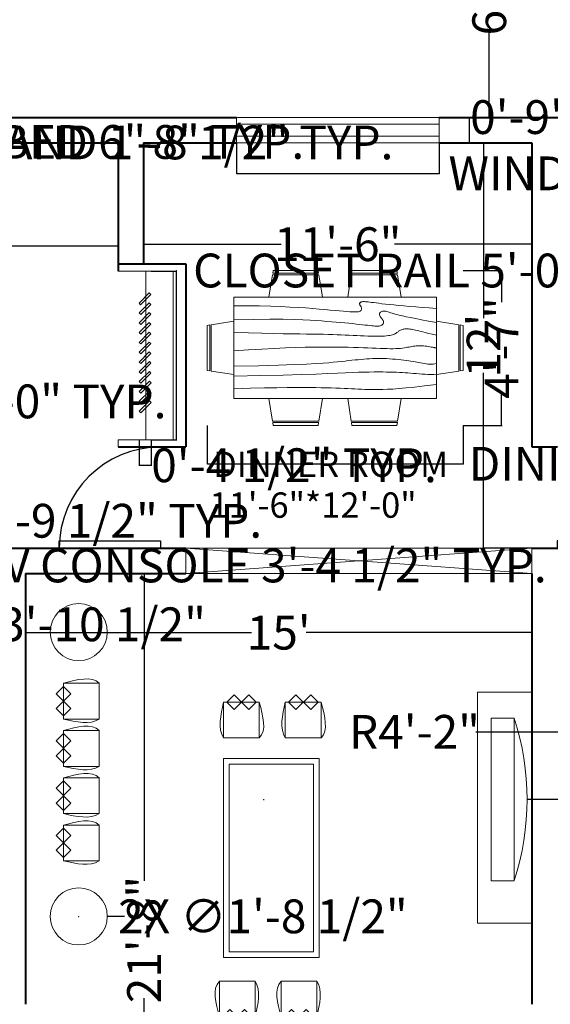
# Model space of a CAD drawing. Units: inches. Extents: x 1146 to 2917, y 889 to 2437.
# Tile 7 of 13: x 1603 to 1792, y 1867 to 2217. Entities that reach past the tile are written whole.
import ezdxf

# ---------------------------------------------------------------- set-up
doc = ezdxf.new("R2010")
doc.units = ezdxf.units.IN
doc.header["$MEASUREMENT"] = 0
for name, color, linetype, lineweight in [('A-ANNO-DIMS', 2, 'Continuous', 18), ('A-AREA-IDEN', 7, 'Continuous', 18), ('A-FLOR-CASE', 9, 'Continuous', 20), ('A-FURN', 9, 'Continuous', 18), ('door', 10, 'Continuous', 25), ('openings', 130, 'Continuous', 18), ('wall', 7, 'Continuous', 40), ('window', 5, 'Continuous', 18)]:
    doc.layers.add(name, color=color, linetype=linetype, lineweight=lineweight)
doc.styles.get("Standard").update_dxf_attribs({"font": 'arial.ttf'})
doc.dimstyles.get("Standard").update_dxf_attribs({"dimtxt": 12, "dimasz": 0.18, "dimexe": 0.18, "dimexo": 0.0625, "dimgap": 0.09, "dimtad": 0, "dimtoh": 1, "dimdec": 1, "dimzin": 0, "dimdsep": 46, "dimlunit": 4, "dimtxsty": 'Standard', "dimcen": 0.09, "dimadec": 0, "dimazin": 0, "dimtfac": 1, "dimtdec": 1, "dimtofl": 0, "dimtmove": 0, "dimatfit": 3, "dimfxl": 1, "dimtolj": 1, "dimtzin": 0, "dimarcsym": 0})

# ---------------------------------------------------------------- blocks, each defined once
blk = doc.blocks.new('*U19')
for p, q in [((0, 0), (0, -6)), ((24, 0), (24, -6))]:
    blk.add_line(p, q)
blk.add_lwpolyline([(0, 0), (0, 24), (1.75, 24), (1.75, 0)], close=True)
blk.add_arc((0, 0), 24, 0, 90)
blk = doc.blocks.new('*U20')
for p, q in [((0, 0), (0, 6)), ((24, 0), (24, 6))]:
    blk.add_line(p, q)
blk.add_lwpolyline([(0, 0), (0, -24), (1.75, -24), (1.75, 0)], close=True)
blk.add_arc((0, 0), 24, 270, 0)
blk = doc.blocks.new('*D24')
at = {"layer": 'A-ANNO-DIMS', "color": 0, "lineweight": -2, "transparency": 16777216}
for p, q in [((1470.13, 2173.33), (1470.13, 2136.54)), ((1638.13, 2173.33), (1638.13, 2136.54)), ((1470.31, 2136.72), (1544.43, 2136.72)), ((1637.95, 2136.72), (1563.84, 2136.72))]:
    blk.add_line(p, q, dxfattribs=at)
at = {"layer": 'A-ANNO-DIMS', "color": 0, "transparency": 16777216}
for points in [[(1470.31, 2136.75), (1470.31, 2136.69), (1470.13, 2136.72)], [(1637.95, 2136.75), (1637.95, 2136.69), (1638.13, 2136.72)]]:
    blk.add_solid(points, dxfattribs=at)
at = {"layer": 'Defpoints', "color": 0, "transparency": 16777216}
for p in [(1470.13, 2173.39), (1638.13, 2173.39), (1638.13, 2136.72)]:
    blk.add_point(p, dxfattribs=at)
at = {"layer": 'A-ANNO-DIMS', "color": 0, "transparency": 16777216, "insert": (1554.13, 2136.72), "char_height": 12, "attachment_point": 5}
blk.add_mtext("\\A1;14'", dxfattribs=at)
blk = doc.blocks.new('*D26')
at = {"layer": 'A-ANNO-DIMS', "color": 0, "lineweight": -2, "transparency": 16777216}
for p, q in [((1785.07, 2173.39), (1767.76, 2173.39)), ((1767.94, 2173.21), (1767.94, 2111.1)), ((1767.94, 2029.57), (1767.94, 2091.68)), ((1785.07, 2029.39), (1767.76, 2029.39))]:
    blk.add_line(p, q, dxfattribs=at)
at = {"layer": 'A-ANNO-DIMS', "color": 0, "transparency": 16777216}
for points in [[(1767.91, 2173.21), (1767.97, 2173.21), (1767.94, 2173.39)], [(1767.91, 2029.57), (1767.97, 2029.57), (1767.94, 2029.39)]]:
    blk.add_solid(points, dxfattribs=at)
at = {"layer": 'Defpoints', "color": 0, "transparency": 16777216}
for p in [(1785.13, 2173.39), (1767.94, 2029.39), (1785.13, 2029.39)]:
    blk.add_point(p, dxfattribs=at)
at = {"layer": 'A-ANNO-DIMS', "color": 0, "transparency": 16777216, "insert": (1767.94, 2101.39), "char_height": 12, "attachment_point": 5, "rotation": 90}
blk.add_mtext("\\A1;12'", dxfattribs=at)
blk = doc.blocks.new('*D27')
at = {"layer": 'A-ANNO-DIMS', "color": 0, "lineweight": -2, "transparency": 16777216}
for p, q in [((1647.13, 2173.33), (1647.13, 2137.25)), ((1785.13, 2173.33), (1785.13, 2137.25)), ((1647.31, 2137.43), (1696, 2137.43)), ((1784.95, 2137.43), (1736.27, 2137.43))]:
    blk.add_line(p, q, dxfattribs=at)
at = {"layer": 'A-ANNO-DIMS', "color": 0, "transparency": 16777216}
for points in [[(1647.31, 2137.46), (1647.31, 2137.4), (1647.13, 2137.43)], [(1784.95, 2137.46), (1784.95, 2137.4), (1785.13, 2137.43)]]:
    blk.add_solid(points, dxfattribs=at)
at = {"layer": 'Defpoints', "color": 0, "transparency": 16777216}
for p in [(1647.13, 2173.39), (1785.13, 2173.39), (1785.13, 2137.43)]:
    blk.add_point(p, dxfattribs=at)
at = {"layer": 'A-ANNO-DIMS', "color": 0, "transparency": 16777216, "insert": (1716.13, 2137.43), "char_height": 12, "attachment_point": 5}
blk.add_mtext('\\A1;11\'-6"', dxfattribs=at)
blk = doc.blocks.new('*D38')
at = {"layer": 'A-ANNO-DIMS', "color": 0, "lineweight": -2, "transparency": 16777216}
for p, q in [((1605.13, 2020.33), (1605.13, 1999.24)), ((1785.13, 2020.33), (1785.13, 1999.24)), ((1605.31, 1999.42), (1685.43, 1999.42)), ((1784.95, 1999.42), (1704.84, 1999.42))]:
    blk.add_line(p, q, dxfattribs=at)
at = {"layer": 'A-ANNO-DIMS', "color": 0, "transparency": 16777216}
for points in [[(1605.31, 1999.45), (1605.31, 1999.39), (1605.13, 1999.42)], [(1784.95, 1999.45), (1784.95, 1999.39), (1785.13, 1999.42)]]:
    blk.add_solid(points, dxfattribs=at)
at = {"layer": 'Defpoints', "color": 0, "transparency": 16777216}
for p in [(1605.13, 2020.39), (1785.13, 2020.39), (1785.13, 1999.42)]:
    blk.add_point(p, dxfattribs=at)
at = {"layer": 'A-ANNO-DIMS', "color": 0, "transparency": 16777216, "insert": (1695.13, 1999.42), "char_height": 12, "attachment_point": 5}
blk.add_mtext("\\A1;15'", dxfattribs=at)
blk = doc.blocks.new('*D39')
at = {"layer": 'A-ANNO-DIMS', "color": 0, "lineweight": -2, "transparency": 16777216}
for p, q in [((1605.2, 2020.39), (1647.47, 2020.39)), ((1647.29, 2020.21), (1647.29, 1911.2)), ((1647.29, 1760.57), (1647.29, 1869.59)), ((1605.2, 1760.39), (1647.47, 1760.39))]:
    blk.add_line(p, q, dxfattribs=at)
at = {"layer": 'A-ANNO-DIMS', "color": 0, "transparency": 16777216}
for points in [[(1647.26, 2020.21), (1647.32, 2020.21), (1647.29, 2020.39)], [(1647.26, 1760.57), (1647.32, 1760.57), (1647.29, 1760.39)]]:
    blk.add_solid(points, dxfattribs=at)
at = {"layer": 'Defpoints', "color": 0, "transparency": 16777216}
for p in [(1605.13, 2020.39), (1605.13, 1760.39), (1647.29, 1760.39)]:
    blk.add_point(p, dxfattribs=at)
at = {"layer": 'A-ANNO-DIMS', "color": 0, "transparency": 16777216, "insert": (1647.29, 1890.39), "char_height": 12, "attachment_point": 5, "rotation": 90}
blk.add_mtext('\\A1;21\'-8"', dxfattribs=at)
blk = doc.blocks.new('Dining Set - 36 x 72 in.')
for p, q in [((-22.2343, 26.00059), (-23.4847, 17.99762)), ((-22.2304, 26), (-5.7608, 26)), ((-22, 27.5), (-22.1562, 26.50042)), ((-5.8416, 26.5), (-22.1534, 26.5)), ((-22, 27.5), (-6, 27.5)), ((-5.8437, 26.49966), (-6, 27.5)), ((-4.5152, 17.99762), (-5.7655, 25.99926)), ((5.7657, 26.00059), (4.5153, 17.99762)), ((5.7696, 26), (22.2392, 26)), ((6, 27.5), (5.8438, 26.50042)), ((22.1584, 26.5), (5.8466, 26.5)), ((6, 27.5), (22, 27.5)), ((22.1563, 26.49966), (22, 27.5)), ((23.4848, 17.99762), (22.2345, 25.99926)), ((36, 18), (-36, 18)), ((-36, 18), (-36, -18)), ((36, -18), (36, 18)), ((-45.5, 8), (-44.5004, 8.15617)), ((-45.5, 8), (-45.5, -8)), ((-44.5, -8.15843), (-44.5, 8.15338)), ((-44.0006, 8.23428), (-35.9976, 9.48474)), ((-44, 8.23041), (-44, -8.23915)), ((44.0006, 8.23428), (35.9976, 9.48474)), ((44, 8.23041), (44, -8.23915)), ((44.5, -8.15843), (44.5, 8.15338)), ((45.5, 8), (44.5005, 8.15617)), ((45.5, 8), (45.5, -8)), ((-44.4997, -8.15631), (-45.5, -8)), ((-35.9976, -9.48476), (-43.9993, -8.2345)), ((35.9976, -9.48476), (43.9993, -8.2345)), ((44.4997, -8.15631), (45.5, -8)), ((-36, -18), (36, -18)), ((-22.2343, -26.0006), (-23.4847, -17.99762)), ((-4.5152, -17.99762), (-5.7655, -25.99928)), ((5.7657, -26.0006), (4.5153, -17.99762)), ((23.4848, -17.99762), (22.2345, -25.99928)), ((-22.2304, -26), (-5.7608, -26)), ((-22, -27.5), (-22.1562, -26.50044)), ((-5.8416, -26.5), (-22.1534, -26.5)), ((-22, -27.5), (-6, -27.5)), ((-5.8437, -26.49967), (-6, -27.5)), ((5.7696, -26), (22.2392, -26)), ((6, -27.5), (5.8438, -26.50044)), ((22.1584, -26.5), (5.8466, -26.5)), ((6, -27.5), (22, -27.5)), ((22.1563, -26.49967), (22, -27.5))]:
    blk.add_line(p, q)
for points in [[(-36, 15), (-31.1772, 14.97754), (-26.8079, 14.91406), (-22.8538, 14.81543), (-19.276, 14.6875), (-16.0362, 14.53613), (-13.0957, 14.36718), (-10.4159, 14.18652), (-7.9583, 14), (-5.6904, 13.81315), (-3.6035, 13.63021), (-1.6954, 13.45508), (0.0365, 13.29166), (1.5945, 13.14388), (2.9811, 13.01562), (4.1988, 12.9108), (5.25, 12.83333), (6.1393, 12.78613), (6.8802, 12.76823), (7.4883, 12.77767), (7.9792, 12.8125), (8.3685, 12.87077), (8.6719, 12.95052), (8.9049, 13.0498), (9.0833, 13.16666), (9.2205, 13.29899), (9.3216, 13.44401), (9.3895, 13.59879), (9.4271, 13.76041), (9.4373, 13.92594), (9.4232, 14.09245), (9.3875, 14.257), (9.3333, 14.41666), (9.2638, 14.56917), (9.1836, 14.71484), (9.0975, 14.85465), (9.0104, 14.98958), (8.9272, 15.1206), (8.8529, 15.2487), (8.7922, 15.37483), (8.75, 15.5), (8.7305, 15.62467), (8.7344, 15.74739), (8.7617, 15.86621), (8.8125, 15.97916), (8.8867, 16.08431), (8.9844, 16.17968), (9.1055, 16.26334), (9.25, 16.33333), (9.4189, 16.38802), (9.6172, 16.42708), (9.8506, 16.45052), (10.125, 16.45833), (10.4463, 16.45052), (10.8203, 16.42708), (11.2529, 16.38802), (11.75, 16.33333), (12.3184, 16.26318), (12.9694, 16.17838), (13.7151, 16.07991), (14.5677, 15.96875), (15.5395, 15.84586), (16.6426, 15.71224), (17.8893, 15.56884), (19.2917, 15.41666), (20.859, 15.25667), (22.5879, 15.08984), (24.4721, 14.91715), (26.5052, 14.73958), (28.6809, 14.5581), (30.9929, 14.3737), (33.4347, 14.18733), (36, 14)], [(-36, 10), (-28.9766, 10.14274), (-23.1725, 10.20442), (-18.4241, 10.19775), (-14.5677, 10.13541), (-11.4399, 10.03011), (-8.877, 9.89453), (-6.7154, 9.74137), (-4.7917, 9.58333), (-2.9698, 9.43082), (-1.2246, 9.28515), (0.4415, 9.14534), (2.026, 9.01041), (3.5266, 8.87939), (4.9408, 8.7513), (6.266, 8.62516), (7.5, 8.5), (8.6411, 8.37549), (9.6914, 8.2539), (10.6538, 8.13818), (11.5312, 8.03125), (12.3267, 7.93603), (13.043, 7.85547), (13.6831, 7.79248), (14.25, 7.75), (14.7471, 7.7303), (15.1797, 7.73307), (15.5537, 7.75732), (15.875, 7.80208), (16.1494, 7.86637), (16.3828, 7.94922), (16.5811, 8.04964), (16.75, 8.16666), (16.8944, 8.29915), (17.0143, 8.44531), (17.1089, 8.60319), (17.1771, 8.77083), (17.218, 8.94629), (17.2305, 9.1276), (17.2137, 9.31282), (17.1667, 9.5), (17.0895, 9.6875), (16.987, 9.875), (16.8649, 10.0625), (16.7292, 10.25), (16.5856, 10.4375), (16.4401, 10.625), (16.2985, 10.8125), (16.1667, 11), (16.05, 11.18733), (15.9518, 11.3737), (15.8752, 11.5581), (15.8229, 11.73958), (15.798, 11.91715), (15.8034, 12.08984), (15.842, 12.25667), (15.9167, 12.41666), (16.0295, 12.56836), (16.1784, 12.70833), (16.3605, 12.83268), (16.5729, 12.9375), (16.8127, 13.01888), (17.0768, 13.07291), (17.3625, 13.0957), (17.6667, 13.08333), (17.9894, 13.03312), (18.3418, 12.94726), (18.7382, 12.82918), (19.1927, 12.68229), (19.7195, 12.51001), (20.3327, 12.31575), (21.0465, 12.10294), (21.875, 11.875), (22.8357, 11.63354), (23.959, 11.37304), (25.2786, 11.08618), (26.8282, 10.76562), (28.6414, 10.40405), (30.752, 9.99414), (33.1936, 9.52856), (36, 9)], [(-36, 5.5), (-30.7157, 5.3348), (-26.069, 5.20963), (-21.9946, 5.11767), (-18.4271, 5.05208), (-15.3009, 5.00602), (-12.5508, 4.97265), (-10.1112, 4.94515), (-7.9167, 4.91666), (-5.909, 4.88167), (-4.0586, 4.83984), (-2.3429, 4.79215), (-0.7396, 4.73958), (0.7739, 4.6831), (2.22, 4.6237), (3.6213, 4.56233), (5, 4.5), (6.373, 4.43782), (7.7344, 4.3776), (9.0723, 4.32129), (10.375, 4.27083), (11.6309, 4.22819), (12.8281, 4.19531), (13.9551, 4.17415), (15, 4.16666), (15.954, 4.17448), (16.819, 4.19791), (17.6001, 4.23698), (18.3021, 4.29166), (18.9299, 4.36198), (19.4883, 4.44791), (19.9823, 4.54948), (20.4167, 4.66666), (20.7969, 4.79899), (21.1302, 4.94401), (21.4245, 5.09879), (21.6875, 5.26041), (21.9271, 5.42594), (22.1511, 5.59245), (22.3672, 5.757), (22.5834, 5.91666), (22.8065, 6.06868), (23.0404, 6.21093), (23.2879, 6.34147), (23.5521, 6.45833), (23.8358, 6.55957), (24.142, 6.64323), (24.4735, 6.70735), (24.8334, 6.75), (25.2235, 6.76969), (25.642, 6.76692), (26.0858, 6.74267), (26.5521, 6.69791), (27.0379, 6.63362), (27.5404, 6.55078), (28.0565, 6.45036), (28.5834, 6.33333), (29.1242, 6.19987), (29.7071, 6.04687), (30.3661, 5.87044), (31.1354, 5.66666), (32.0493, 5.43164), (33.142, 5.16146), (34.4475, 4.85221), (36, 4.5)], [(-36, -1), (-30.7915, -0.6591), (-26.0195, -0.38216), (-21.6519, -0.16284), (-17.6563, 0.00521), (-14.0005, 0.12833), (-10.6523, 0.21289), (-7.5796, 0.26522), (-4.75, 0.29166), (-2.134, 0.29793), (0.2878, 0.28711), (2.5317, 0.26163), (4.6146, 0.22396), (6.5529, 0.17651), (8.3633, 0.12174), (10.0623, 0.06209), (11.6667, 0), (13.1899, -0.06201), (14.6341, -0.1211), (15.9982, -0.17432), (17.2813, -0.21875), (18.4823, -0.25147), (19.6003, -0.26953), (20.6343, -0.27002), (21.5834, -0.25), (22.4481, -0.20768), (23.2357, -0.14584), (23.9549, -0.06836), (24.6146, 0.02083), (25.2235, 0.11784), (25.7904, 0.21875), (26.3241, 0.31966), (26.8334, 0.41666), (27.3265, 0.50618), (27.8099, 0.58593), (28.2894, 0.65397), (28.7709, 0.70833), (29.2601, 0.74707), (29.763, 0.76823), (30.2855, 0.76985), (30.8334, 0.75), (31.4088, 0.70784), (31.9994, 0.64713), (32.589, 0.57275), (33.1615, 0.48958), (33.7008, 0.4025), (34.1908, 0.3164), (34.6153, 0.23616), (34.9584, 0.16666), (35.2099, 0.11165), (35.3848, 0.07031), (35.504, 0.04069), (35.5886, 0.02083), (35.6594, 0.00879), (35.7377, 0.0026), (35.8442, 0.00032), (36, 0)], [(-36, -6.5), (-27.1843, -6.31267), (-20.084, -6.1263), (-14.469, -5.9419), (-10.1094, -5.76042), (-6.7752, -5.58285), (-4.2363, -5.41016), (-2.2629, -5.24333), (-0.625, -5.08334), (0.8708, -4.93099), (2.2715, -4.78646), (3.5872, -4.64974), (4.8281, -4.52084), (6.0046, -4.39974), (7.127, -4.28646), (8.2053, -4.18099), (9.25, -4.08334), (10.2705, -3.99382), (11.2734, -3.91407), (12.2647, -3.84603), (13.25, -3.79167), (14.2354, -3.75293), (15.2266, -3.73177), (16.2295, -3.73015), (17.25, -3.75), (18.2912, -3.79248), (19.3451, -3.85547), (20.4009, -3.93604), (21.4479, -4.03125), (22.4754, -4.13819), (23.4727, -4.25391), (24.4289, -4.37549), (25.3334, -4.5), (26.1785, -4.62492), (26.9694, -4.74935), (27.7145, -4.87281), (28.4219, -4.99479), (29.1, -5.11483), (29.7572, -5.23242), (30.4016, -5.34709), (31.0417, -5.45834), (31.6837, -5.56437), (32.3262, -5.65821), (32.9658, -5.73153), (33.599, -5.77604), (34.2224, -5.78345), (34.8327, -5.74545), (35.4264, -5.65373), (36, -5.5)], [(-36, -10), (-26.4022, -9.81299), (-18.4675, -9.62891), (-11.9839, -9.45069), (-6.7396, -9.28125), (-2.5226, -9.12354), (0.8789, -8.98047), (3.6769, -8.85498), (6.0833, -8.75), (8.2767, -8.66765), (10.3021, -8.60677), (12.1712, -8.56543), (13.8958, -8.54167), (15.4876, -8.53353), (16.9583, -8.53907), (18.3197, -8.55632), (19.5834, -8.58334), (20.7616, -8.61841), (21.8685, -8.66081), (22.9188, -8.71004), (23.9271, -8.76563), (24.9081, -8.82707), (25.8763, -8.89388), (26.8465, -8.96558), (27.8334, -9.04167), (28.8474, -9.12118), (29.8828, -9.20117), (30.93, -9.27824), (31.9792, -9.34896), (33.0205, -9.40991), (34.0443, -9.45768), (35.0407, -9.48885), (36, -9.5)], [(-36, -14.5), (-30.0881, -14.33513), (-25.0332, -14.21224), (-20.7312, -14.12647), (-17.0781, -14.07292), (-13.97, -14.04671), (-11.3027, -14.04297), (-8.9724, -14.05681), (-6.875, -14.08334), (-4.9224, -14.11833), (-3.0905, -14.16016), (-1.3709, -14.20785), (0.2448, -14.26042), (1.7647, -14.3169), (3.1973, -14.3763), (4.5507, -14.43767), (5.8333, -14.5), (7.0554, -14.5621), (8.235, -14.62175), (9.3922, -14.67652), (10.5469, -14.72396), (11.7192, -14.76164), (12.929, -14.78711), (14.1965, -14.79794), (15.5417, -14.79167), (16.9933, -14.76424), (18.6152, -14.70508), (20.4804, -14.60197), (22.6615, -14.44271), (25.2312, -14.21509), (28.2624, -13.9069), (31.8277, -13.50594), (36, -13)]]:
    blk.add_lwpolyline(points)
blk = doc.blocks.new('*D50')
at = {"layer": 'A-ANNO-DIMS', "color": 0, "lineweight": -2, "transparency": 16777216}
for p, q in [((1773.07, 2254.39), (1769.77, 2254.39)), ((1769.95, 2254.21), (1769.95, 2224.04)), ((1769.95, 2182.57), (1769.95, 2212.75)), ((1773.07, 2182.39), (1769.77, 2182.39))]:
    blk.add_line(p, q, dxfattribs=at)
at = {"layer": 'A-ANNO-DIMS', "color": 0, "transparency": 16777216}
for points in [[(1769.92, 2254.21), (1769.98, 2254.21), (1769.95, 2254.39)], [(1769.92, 2182.57), (1769.98, 2182.57), (1769.95, 2182.39)]]:
    blk.add_solid(points, dxfattribs=at)
at = {"layer": 'Defpoints', "color": 0, "transparency": 16777216}
for p in [(1773.13, 2254.39), (1769.95, 2182.39), (1773.13, 2182.39)]:
    blk.add_point(p, dxfattribs=at)
at = {"layer": 'A-ANNO-DIMS', "color": 0, "transparency": 16777216, "insert": (1769.95, 2218.39), "char_height": 12, "attachment_point": 5, "rotation": 90}
blk.add_mtext("\\A1;6'", dxfattribs=at)
blk = doc.blocks.new('CHAIR-LOUNGE')
blk.add_line((0, 8.98), (8.98, 0))
blk.add_lwpolyline([(0, 8.98), (8.98, 17.96), (17.96, 8.98), (8.98, 0)])
for points in [[(9.79, 17.15), (13.47, 17.15), (13.47, 13.47), (9.79, 13.47)], [(13.52, 13.42), (17.2, 13.42), (17.2, 9.74), (13.52, 9.74)]]:
    blk.add_lwpolyline(points, close=True)
for points in [[(8.98, 17.96), (4.93, 15.41), (0.87, 12.85), (0, 8.98)], [(17.96, 8.98), (15.38, 4.49), (12.8, -0.01), (8.98, 0)]]:
    blk.add_open_spline(points, degree=3)
blk = doc.blocks.new('WINDOW-PLAN-72-2')
for points in [[(0, 9), (72, 9), (72, 0), (0, 0)], [(0, 6.65), (72, 6.65), (72, 2.45), (0, 2.45)]]:
    blk.add_lwpolyline(points, close=True)
blk = doc.blocks.new('CLOSET-RAIL-HANGERS')
blk.add_line((2.37, 60), (2.37, 0))
for points in [[(0, 48.59), (3.61, 52.2), (4.18, 51.63), (0.57, 48.02)], [(0.01, 45.11), (3.62, 48.71), (4.18, 48.15), (0.58, 44.54)], [(0.02, 41.62), (3.62, 45.23), (4.19, 44.66), (0.59, 41.05)], [(0.02, 38.13), (3.63, 41.74), (4.2, 41.17), (0.59, 37.56)], [(0.03, 34.65), (3.64, 38.25), (4.21, 37.69), (0.6, 34.08)], [(0.04, 31.16), (3.65, 34.77), (4.22, 34.2), (0.61, 30.59)], [(0.05, 27.67), (3.65, 31.28), (4.22, 30.71), (0.62, 27.1)], [(0.06, 24.19), (3.66, 27.8), (4.23, 27.23), (0.62, 23.62)], [(0.06, 20.7), (3.67, 24.31), (4.24, 23.74), (0.63, 20.13)], [(0.07, 17.21), (3.68, 20.82), (4.25, 20.25), (0.64, 16.65)], [(0.08, 13.73), (3.69, 17.34), (4.26, 16.77), (0.65, 13.16)], [(0.09, 10.24), (3.69, 13.85), (4.26, 13.28), (0.66, 9.67)]]:
    blk.add_lwpolyline(points, close=True)
blk = doc.blocks.new('*D99')
at = {"layer": 'A-ANNO-DIMS', "color": 0, "lineweight": -2, "transparency": 16777216}
for p, q in [((1521.84, 2173.39), (1525.02, 2173.39)), ((1524.84, 2173.39), (1524.84, 2173.57)), ((1524.84, 2173.57), (1525.02, 2173.57)), ((1524.84, 2153.21), (1524.84, 2173.21)), ((1521.84, 2153.03), (1525.02, 2153.03))]:
    blk.add_line(p, q, dxfattribs=at)
at = {"layer": 'A-ANNO-DIMS', "color": 0, "transparency": 16777216}
for points in [[(1524.81, 2173.21), (1524.87, 2173.21), (1524.84, 2173.39)], [(1524.81, 2153.21), (1524.87, 2153.21), (1524.84, 2153.03)]]:
    blk.add_solid(points, dxfattribs=at)
at = {"layer": 'Defpoints', "color": 0, "transparency": 16777216}
for p in [(1521.78, 2173.39), (1524.84, 2173.39), (1521.78, 2153.03)]:
    blk.add_point(p, dxfattribs=at)
at = {"layer": 'A-ANNO-DIMS', "color": 0, "transparency": 16777216, "insert": (1632.18, 2173.57), "char_height": 12, "attachment_point": 5}
blk.add_mtext('\\A1;NIGHTSTAND 1\'-8 1/2" TYP.', dxfattribs=at)
blk = doc.blocks.new('*D101')
at = {"layer": 'A-ANNO-DIMS', "color": 0, "lineweight": -2, "transparency": 16777216}
for p, q in [((1581.84, 2173.57), (1593.96, 2173.57)), ((1593.78, 2173.57), (1593.78, 2173.75)), ((1593.78, 2173.75), (1593.96, 2173.75)), ((1593.78, 2093.75), (1593.78, 2173.39)), ((1581.84, 2093.57), (1593.96, 2093.57))]:
    blk.add_line(p, q, dxfattribs=at)
at = {"layer": 'A-ANNO-DIMS', "color": 0, "transparency": 16777216}
for points in [[(1593.75, 2173.39), (1593.81, 2173.39), (1593.78, 2173.57)], [(1593.75, 2093.75), (1593.81, 2093.75), (1593.78, 2093.57)]]:
    blk.add_solid(points, dxfattribs=at)
at = {"layer": 'Defpoints', "color": 0, "transparency": 16777216}
for p in [(1581.78, 2173.57), (1593.78, 2173.57), (1581.78, 2093.57)]:
    blk.add_point(p, dxfattribs=at)
at = {"layer": 'A-ANNO-DIMS', "color": 0, "transparency": 16777216, "insert": (1649.92, 2173.75), "char_height": 12, "attachment_point": 5}
blk.add_mtext('\\A1;BED 6\'-8" TYP.', dxfattribs=at)
blk = doc.blocks.new('*D102')
at = {"layer": 'A-ANNO-DIMS', "color": 0, "lineweight": -2, "transparency": 16777216}
for p, q in [((1521.78, 2093.51), (1521.78, 2081.39)), ((1581.78, 2093.51), (1581.78, 2081.39)), ((1521.96, 2081.57), (1581.6, 2081.57)), ((1581.78, 2081.57), (1581.96, 2081.57))]:
    blk.add_line(p, q, dxfattribs=at)
at = {"layer": 'A-ANNO-DIMS', "color": 0, "transparency": 16777216}
for points in [[(1521.96, 2081.6), (1521.96, 2081.54), (1521.78, 2081.57)], [(1581.6, 2081.6), (1581.6, 2081.54), (1581.78, 2081.57)]]:
    blk.add_solid(points, dxfattribs=at)
at = {"layer": 'Defpoints', "color": 0, "transparency": 16777216}
for p in [(1521.78, 2093.57), (1581.78, 2093.57), (1581.78, 2081.57)]:
    blk.add_point(p, dxfattribs=at)
at = {"layer": 'A-ANNO-DIMS', "color": 0, "transparency": 16777216, "insert": (1618.62, 2081.57), "char_height": 12, "attachment_point": 5}
blk.add_mtext('\\A1;5\'-0" TYP.', dxfattribs=at)
blk = doc.blocks.new('*D105')
at = {"layer": 'A-ANNO-DIMS', "color": 0, "lineweight": -2, "transparency": 16777216}
for p, q in [((1649.84, 2127.89), (1658.95, 2127.89)), ((1658.77, 2127.89), (1658.77, 2128.07)), ((1658.77, 2128.07), (1658.95, 2128.07)), ((1658.77, 2068.07), (1658.77, 2127.71)), ((1649.84, 2067.89), (1658.95, 2067.89))]:
    blk.add_line(p, q, dxfattribs=at)
at = {"layer": 'A-ANNO-DIMS', "color": 0, "transparency": 16777216}
for points in [[(1658.74, 2127.71), (1658.8, 2127.71), (1658.77, 2127.89)], [(1658.74, 2068.07), (1658.8, 2068.07), (1658.77, 2067.89)]]:
    blk.add_solid(points, dxfattribs=at)
at = {"layer": 'Defpoints', "color": 0, "transparency": 16777216}
for p in [(1649.77, 2127.89), (1658.77, 2127.89), (1649.77, 2067.89)]:
    blk.add_point(p, dxfattribs=at)
at = {"layer": 'A-ANNO-DIMS', "color": 0, "transparency": 16777216, "insert": (1752.38, 2128.07), "char_height": 12, "attachment_point": 5}
blk.add_mtext('\\A1;CLOSET RAIL 5\'-0" TYP.', dxfattribs=at)
blk = doc.blocks.new('*D106')
at = {"layer": 'A-ANNO-DIMS', "color": 0, "lineweight": -2, "transparency": 16777216}
for p, q in [((1645.51, 2067.83), (1645.51, 2058.71)), ((1649.77, 2067.83), (1649.77, 2058.71)), ((1645.69, 2058.89), (1649.59, 2058.89)), ((1649.77, 2058.89), (1649.95, 2058.89))]:
    blk.add_line(p, q, dxfattribs=at)
at = {"layer": 'A-ANNO-DIMS', "color": 0, "transparency": 16777216}
for points in [[(1645.69, 2058.92), (1645.69, 2058.86), (1645.51, 2058.89)], [(1649.59, 2058.92), (1649.59, 2058.86), (1649.77, 2058.89)]]:
    blk.add_solid(points, dxfattribs=at)
at = {"layer": 'Defpoints', "color": 0, "transparency": 16777216}
for p in [(1645.51, 2067.89), (1649.77, 2067.89), (1649.77, 2058.89)]:
    blk.add_point(p, dxfattribs=at)
at = {"layer": 'A-ANNO-DIMS', "color": 0, "transparency": 16777216, "insert": (1700.6, 2058.89), "char_height": 12, "attachment_point": 5}
blk.add_mtext('\\A1;0\'-4 1/2" TYP.', dxfattribs=at)
blk = doc.blocks.new('*D109')
at = {"layer": 'A-ANNO-DIMS', "color": 0, "lineweight": -2, "transparency": 16777216}
for p, q in [((1540.88, 2029.33), (1540.88, 2023.11)), ((1581.59, 2029.33), (1581.59, 2023.11)), ((1541.06, 2023.29), (1581.41, 2023.29)), ((1581.59, 2023.29), (1581.77, 2023.29))]:
    blk.add_line(p, q, dxfattribs=at)
at = {"layer": 'A-ANNO-DIMS', "color": 0, "transparency": 16777216}
for points in [[(1541.06, 2023.32), (1541.06, 2023.26), (1540.88, 2023.29)], [(1581.41, 2023.32), (1581.41, 2023.26), (1581.59, 2023.29)]]:
    blk.add_solid(points, dxfattribs=at)
at = {"layer": 'Defpoints', "color": 0, "transparency": 16777216}
for p in [(1540.88, 2029.39), (1581.59, 2029.39), (1581.59, 2023.29)]:
    blk.add_point(p, dxfattribs=at)
at = {"layer": 'A-ANNO-DIMS', "color": 0, "transparency": 16777216, "insert": (1688.92, 2023.29), "char_height": 12, "attachment_point": 5}
blk.add_mtext('\\A1;TV CONSOLE 3\'-4 1/2" TYP.', dxfattribs=at)
blk = doc.blocks.new('*D110')
at = {"layer": 'A-ANNO-DIMS', "color": 0, "lineweight": -2, "transparency": 16777216}
for p, q in [((1581.65, 2038.99), (1587.87, 2038.99)), ((1587.69, 2038.99), (1587.69, 2039.17)), ((1587.69, 2039.17), (1587.87, 2039.17)), ((1587.69, 2029.57), (1587.69, 2038.81)), ((1581.65, 2029.39), (1587.87, 2029.39))]:
    blk.add_line(p, q, dxfattribs=at)
at = {"layer": 'A-ANNO-DIMS', "color": 0, "transparency": 16777216}
for points in [[(1587.66, 2038.81), (1587.72, 2038.81), (1587.69, 2038.99)], [(1587.66, 2029.57), (1587.72, 2029.57), (1587.69, 2029.39)]]:
    blk.add_solid(points, dxfattribs=at)
at = {"layer": 'Defpoints', "color": 0, "transparency": 16777216}
for p in [(1581.59, 2038.99), (1587.69, 2038.99), (1581.59, 2029.39)]:
    blk.add_point(p, dxfattribs=at)
at = {"layer": 'A-ANNO-DIMS', "color": 0, "transparency": 16777216, "insert": (1638.52, 2039.17), "char_height": 12, "attachment_point": 5}
blk.add_mtext('\\A1;0\'-9 1/2" TYP.', dxfattribs=at)
blk = doc.blocks.new('*D111')
at = {"layer": 'A-ANNO-DIMS', "color": 0, "lineweight": -2, "transparency": 16777216}
for p, q in [((1680.13, 2173.33), (1680.13, 2162.41)), ((1752.13, 2173.33), (1752.13, 2162.41)), ((1680.31, 2162.59), (1751.95, 2162.59)), ((1752.13, 2162.59), (1752.31, 2162.59))]:
    blk.add_line(p, q, dxfattribs=at)
at = {"layer": 'A-ANNO-DIMS', "color": 0, "transparency": 16777216}
for points in [[(1680.31, 2162.62), (1680.31, 2162.56), (1680.13, 2162.59)], [(1751.95, 2162.62), (1751.95, 2162.56), (1752.13, 2162.59)]]:
    blk.add_solid(points, dxfattribs=at)
at = {"layer": 'Defpoints', "color": 0, "transparency": 16777216}
for p in [(1680.13, 2173.39), (1752.13, 2173.39), (1752.13, 2162.59)]:
    blk.add_point(p, dxfattribs=at)
at = {"layer": 'A-ANNO-DIMS', "color": 0, "transparency": 16777216, "insert": (1828.33, 2162.59), "char_height": 12, "attachment_point": 5}
blk.add_mtext('\\A1;WINDOW 6\'-0" TYP.', dxfattribs=at)
blk = doc.blocks.new('*D112')
at = {"layer": 'A-ANNO-DIMS', "color": 0, "lineweight": -2, "transparency": 16777216}
for p, q in [((1752.2, 2182.39), (1763.11, 2182.39)), ((1762.93, 2182.39), (1762.93, 2182.57)), ((1762.93, 2182.57), (1763.11, 2182.57)), ((1762.93, 2173.57), (1762.93, 2182.21)), ((1752.2, 2173.39), (1763.11, 2173.39))]:
    blk.add_line(p, q, dxfattribs=at)
at = {"layer": 'A-ANNO-DIMS', "color": 0, "transparency": 16777216}
for points in [[(1762.9, 2182.21), (1762.96, 2182.21), (1762.93, 2182.39)], [(1762.9, 2173.57), (1762.96, 2173.57), (1762.93, 2173.39)]]:
    blk.add_solid(points, dxfattribs=at)
at = {"layer": 'Defpoints', "color": 0, "transparency": 16777216}
for p in [(1752.13, 2182.39), (1762.93, 2182.39), (1752.13, 2173.39)]:
    blk.add_point(p, dxfattribs=at)
at = {"layer": 'A-ANNO-DIMS', "color": 0, "transparency": 16777216, "insert": (1799.78, 2182.57), "char_height": 12, "attachment_point": 5}
blk.add_mtext('\\A1;0\'-9" TYP.', dxfattribs=at)
blk = doc.blocks.new('*D119')
at = {"layer": 'A-ANNO-DIMS', "color": 0, "lineweight": -2, "transparency": 16777216}
for p, q in [((1669.67, 2073), (1669.67, 2059.24)), ((1760.67, 2073), (1760.67, 2059.24)), ((1669.85, 2059.42), (1760.49, 2059.42)), ((1760.67, 2059.42), (1760.85, 2059.42))]:
    blk.add_line(p, q, dxfattribs=at)
at = {"layer": 'A-ANNO-DIMS', "color": 0, "transparency": 16777216}
for points in [[(1669.85, 2059.45), (1669.85, 2059.39), (1669.67, 2059.42)], [(1760.49, 2059.45), (1760.49, 2059.39), (1760.67, 2059.42)]]:
    blk.add_solid(points, dxfattribs=at)
at = {"layer": 'Defpoints', "color": 0, "transparency": 16777216}
for p in [(1669.67, 2073.07), (1760.67, 2073.07), (1760.67, 2059.42)]:
    blk.add_point(p, dxfattribs=at)
at = {"layer": 'A-ANNO-DIMS', "color": 0, "transparency": 16777216, "insert": (1826.89, 2059.42), "char_height": 12, "attachment_point": 5}
blk.add_mtext('\\A1;DINING SET 7\'-7"', dxfattribs=at)
blk = doc.blocks.new('*D120')
at = {"layer": 'A-ANNO-DIMS', "color": 0, "lineweight": -2, "transparency": 16777216}
for p, q in [((1760.74, 2128.07), (1774.5, 2128.07)), ((1774.32, 2127.89), (1774.32, 2116.85)), ((1774.32, 2073.25), (1774.32, 2084.28)), ((1760.74, 2073.07), (1774.5, 2073.07))]:
    blk.add_line(p, q, dxfattribs=at)
at = {"layer": 'A-ANNO-DIMS', "color": 0, "transparency": 16777216}
for points in [[(1774.29, 2127.89), (1774.35, 2127.89), (1774.32, 2128.07)], [(1774.29, 2073.25), (1774.35, 2073.25), (1774.32, 2073.07)]]:
    blk.add_solid(points, dxfattribs=at)
at = {"layer": 'Defpoints', "color": 0, "transparency": 16777216}
for p in [(1760.67, 2128.07), (1774.32, 2128.07), (1760.67, 2073.07)]:
    blk.add_point(p, dxfattribs=at)
at = {"layer": 'A-ANNO-DIMS', "color": 0, "transparency": 16777216, "insert": (1774.32, 2100.57), "char_height": 12, "attachment_point": 5, "rotation": 90}
blk.add_mtext('\\A1;4\'-7"', dxfattribs=at)
blk = doc.blocks.new('*D168')
at = {"layer": 'A-ANNO-DIMS', "color": 0, "lineweight": -2, "transparency": 16777216}
for p, q in [((1431.13, 2029.45), (1431.13, 2426.57)), ((1431.31, 2426.39), (1674.19, 2426.39)), ((1958.95, 2426.39), (1716.08, 2426.39)), ((1959.13, 2029.45), (1959.13, 2426.57))]:
    blk.add_line(p, q, dxfattribs=at)
at = {"layer": 'A-ANNO-DIMS', "color": 0, "transparency": 16777216}
for points in [[(1431.31, 2426.42), (1431.31, 2426.36), (1431.13, 2426.39)], [(1958.95, 2426.42), (1958.95, 2426.36), (1959.13, 2426.39)]]:
    blk.add_solid(points, dxfattribs=at)
at = {"layer": 'Defpoints', "color": 0, "transparency": 16777216}
for p in [(1959.13, 2426.39), (1431.13, 2029.39), (1959.13, 2029.39)]:
    blk.add_point(p, dxfattribs=at)
at = {"layer": 'A-ANNO-DIMS', "color": 0, "transparency": 16777216, "insert": (1695.13, 2426.39), "char_height": 12, "attachment_point": 5}
blk.add_mtext('\\A1;44\'-0"', dxfattribs=at)
blk = doc.blocks.new('*D175')
at = {"layer": 'A-ANNO-DIMS', "color": 0, "lineweight": -2, "transparency": 16777216}
for p, q in [((1689.74, 1940.2), (1689.92, 1940.2)), ((1689.83, 1940.11), (1689.83, 1940.29)), ((1839.56, 1940.2), (1783.59, 1940.2))]:
    blk.add_line(p, q, dxfattribs=at)
at = {"layer": 'A-ANNO-DIMS', "color": 0, "transparency": 16777216}
blk.add_solid([(1783.59, 1940.23), (1783.59, 1940.17), (1783.41, 1940.2)], dxfattribs=at)
at = {"layer": 'Defpoints', "color": 0, "transparency": 16777216}
for p in [(1689.83, 1940.2), (1783.41, 1940.2)]:
    blk.add_point(p, dxfattribs=at)
at = {"layer": 'A-ANNO-DIMS', "color": 0, "transparency": 16777216, "insert": (1875.32, 1940.2), "char_height": 12, "attachment_point": 5}
blk.add_mtext('\\A1;R7\'-9 1/2"', dxfattribs=at)
blk = doc.blocks.new('*D177')
at = {"layer": 'A-ANNO-DIMS', "color": 0, "lineweight": -2, "transparency": 16777216}
for p, q in [((1765.18, 1964.17), (1794.87, 1964.17)), ((1844.75, 1964.17), (1844.93, 1964.17)), ((1844.84, 1964.08), (1844.84, 1964.26))]:
    blk.add_line(p, q, dxfattribs=at)
at = {"layer": 'A-ANNO-DIMS', "color": 0, "transparency": 16777216}
blk.add_solid([(1794.87, 1964.2), (1794.87, 1964.14), (1795.05, 1964.17)], dxfattribs=at)
at = {"layer": 'Defpoints', "color": 0, "transparency": 16777216}
for p in [(1795.05, 1964.17), (1844.84, 1964.17)]:
    blk.add_point(p, dxfattribs=at)
at = {"layer": 'A-ANNO-DIMS', "color": 0, "transparency": 16777216, "insert": (1743.39, 1964.17), "char_height": 12, "attachment_point": 5}
blk.add_mtext('\\A1;R4\'-2"', dxfattribs=at)
blk = doc.blocks.new('*D178')
at = {"layer": 'A-ANNO-DIMS', "color": 0, "lineweight": -2, "transparency": 16777216}
for p, q in [((1562.58, 2076.67), (1562.76, 2076.67)), ((1562.67, 2076.58), (1562.67, 2076.76)), ((1562.67, 2002.39), (1562.67, 2030.07)), ((1562.85, 2002.39), (1562.67, 2002.39))]:
    blk.add_line(p, q, dxfattribs=at)
at = {"layer": 'A-ANNO-DIMS', "color": 0, "transparency": 16777216}
blk.add_solid([(1562.7, 2030.07), (1562.64, 2030.07), (1562.67, 2030.25)], dxfattribs=at)
at = {"layer": 'Defpoints', "color": 0, "transparency": 16777216}
for p in [(1562.67, 2076.67), (1562.67, 2030.25)]:
    blk.add_point(p, dxfattribs=at)
at = {"layer": 'A-ANNO-DIMS', "color": 0, "transparency": 16777216, "insert": (1616.27, 2002.39), "char_height": 12, "attachment_point": 5}
blk.add_mtext('\\A1;2X R3\'-10 1/2"', dxfattribs=at)
blk = doc.blocks.new('*D180')
at = {"layer": 'A-ANNO-DIMS', "color": 0, "lineweight": -2, "transparency": 16777216}
for p, q in [((1623.97, 1898.64), (1624.15, 1898.64)), ((1624.06, 1898.55), (1624.06, 1898.73)), ((1640.31, 1898.64), (1634.4, 1898.64))]:
    blk.add_line(p, q, dxfattribs=at)
at = {"layer": 'A-ANNO-DIMS', "color": 0, "transparency": 16777216}
blk.add_solid([(1634.4, 1898.67), (1634.4, 1898.61), (1634.22, 1898.64)], dxfattribs=at)
at = {"layer": 'Defpoints', "color": 0, "transparency": 16777216}
for p in [(1613.91, 1898.64), (1634.22, 1898.64)]:
    blk.add_point(p, dxfattribs=at)
at = {"layer": 'A-ANNO-DIMS', "color": 0, "transparency": 16777216, "insert": (1689.53, 1898.64), "char_height": 12, "attachment_point": 5}
blk.add_mtext('\\A1;2X ∅1\'-8 1/2"', dxfattribs=at)

msp = doc.modelspace()

# ---------------------------------------------------------------- linework, layer by layer
at = {"layer": 'A-FLOR-CASE'}
for p, q in [((1638.13, 2127.89), (1657.63, 2127.89)), ((1657.63, 2127.89), (1657.63, 2067.89)), ((1638.13, 2067.89), (1657.63, 2067.89)), ((1638.13, 2067.89), (1638.13, 2065.39))]:
    msp.add_line(p, q, dxfattribs=at)
at = {"layer": 'A-FURN'}
for points in [[(1765.79, 1978.32), (1785.13, 1978.32), (1785.13, 1896.26), (1765.79, 1896.26)], [(1770.61, 1969.08), (1778.84, 1969.08), (1778.84, 1911.31), (1770.61, 1911.31)], [(1675.57, 1954.75), (1709.46, 1954.75), (1709.46, 1884.05), (1675.57, 1884.05)], [(1677.57, 1952.75), (1707.46, 1952.75), (1707.46, 1886.05), (1677.57, 1886.05)]]:
    msp.add_lwpolyline(points, close=True, dxfattribs=at)
for centre in [(1624.06, 1999.62), (1624.06, 1898.64)]:
    msp.add_circle(centre, 10.15, dxfattribs=at)
msp.add_arc((1689.83, 1940.2), 93.58, 342.0216, 17.9784, dxfattribs=at)
at = {"layer": 'openings'}
for p, q in [((1662.13, 2029.39), (1662.13, 2020.39)), ((1662.13, 2029.39), (1785.13, 2020.39)), ((1662.13, 2020.39), (1785.13, 2029.39)), ((1785.13, 2029.39), (1662.13, 2029.39)), ((1785.13, 2020.39), (1785.13, 2029.39)), ((1785.13, 2020.39), (1662.13, 2020.39))]:
    msp.add_line(p, q, dxfattribs=at)
at = {"layer": 'wall'}
for p, q in [((1573.38, 2182.39), (1680.13, 2182.39)), ((1752.13, 2182.39), (1821.13, 2182.39)), ((1573.38, 2173.39), (1638.13, 2173.39)), ((1638.13, 2173.39), (1638.13, 2127.89)), ((1647.13, 2173.39), (1647.13, 2130.39)), ((1647.13, 2173.39), (1680.13, 2173.39)), ((1752.13, 2173.39), (1785.13, 2173.39)), ((1785.13, 2173.39), (1785.13, 2065.39)), ((1638.13, 2130.39), (1662.13, 2130.39)), ((1662.13, 2130.39), (1662.13, 2065.39)), ((1638.13, 2065.39), (1662.13, 2065.39)), ((1785.13, 2065.39), (1794.13, 2065.39)), ((1470.13, 2029.39), (1662.13, 2029.39)), ((1785.13, 2029.39), (1920.13, 2029.39)), ((1605.13, 2020.39), (1605.13, 1867.39)), ((1605.13, 2020.39), (1662.13, 2020.39)), ((1785.13, 2020.39), (1785.13, 1867.39))]:
    msp.add_line(p, q, dxfattribs=at)

# ---------------------------------------------------------------- block references
at = {"layer": 'A-FLOR-CASE'}
msp.add_blockref('CLOSET-RAIL-HANGERS', (1645.51, 2067.89), dxfattribs=at)
at = {"layer": 'A-FURN'}
msp.add_blockref('Dining Set - 36 x 72 in.', (1715.17, 2100.57), dxfattribs=at)
for p, rotation in [((1637.69, 1975.07), 135.0000000000008), ((1681.9, 1955.67), 44.99999999999964), ((1703.83, 1955.67), 45.00000000000266), ((1637.69, 1958.28), 134.9999999999988), ((1637.69, 1941.49), 134.9999999999938), ((1637.69, 1924.7), 134.9999999999988), ((1680.42, 1881.94), 224.999999999996), ((1702.35, 1881.94), 224.999999999997)]:
    msp.add_blockref('CHAIR-LOUNGE', p, dxfattribs=dict(at, rotation=rotation))
at = {"layer": 'door', "xscale": 1.499999999999961, "yscale": 1.499999999999961, "zscale": 1.499999999999961, "rotation": 90}
for name, p in [('*U19', (1653.13, 2029.39)), ('*U20', (1794.13, 2029.39))]:
    msp.add_blockref(name, p, dxfattribs=at)
at = {"layer": 'window'}
msp.add_blockref('WINDOW-PLAN-72-2', (1680.13, 2173.39), dxfattribs=at)

# ---------------------------------------------------------------- texts
at = {"layer": 'A-AREA-IDEN', "char_height": 9, "attachment_point": 1}
for s, width, heights, insert in [('DINNER ROOM', 113.337, [0], (1671.8, 2063.75)), ('11\'-6"*12\'-0"', 69.7556, [0.204], (1670.55, 2049.24))]:
    msp.add_mtext_dynamic_manual_height_columns(s, width=width, gutter_width=1, heights=heights, dxfattribs=dict(at, insert=insert))

# ---------------------------------------------------------------- dimensions: what is measured, and where the dimension line sits
at = {"layer": 'A-ANNO-DIMS'}
dim = msp.add_linear_dim(base=(1959.13, 2426.39), p1=(1431.13, 2029.39), p2=(1959.13, 2029.39), dimstyle='Standard', override={"dimdec": 1, "dimlfac": 1, "dimrnd": 0, "dimzin": 1, "dimdsep": 46, "dimlunit": 4, "dimfrac": 2}, dxfattribs=at)
dim.commit()
dim.dimension.update_dxf_attribs({"geometry": '*D168', "text_midpoint": (1695.13, 2426.39)})
for p1, p2, distance, picture, middle in [((1773.13, 2254.39), (1773.13, 2182.39), -3.19, '*D50', (1769.95, 2218.39)), ((1470.13, 2173.39), (1638.13, 2173.39), -36.67, '*D24', (1554.13, 2136.72)), ((1647.13, 2173.39), (1785.13, 2173.39), -35.96, '*D27', (1716.13, 2137.43)), ((1605.13, 2020.39), (1605.13, 1760.39), 42.15, '*D39', (1647.29, 1890.39))]:
    dim = msp.add_aligned_dim(p1=p1, p2=p2, distance=distance, dimstyle='Standard', override={"dimclrd": 0, "dimclre": 0, "dimclrt": 0}, dxfattribs=at)
    dim.commit()
    dim.dimension.update_dxf_attribs({"geometry": picture, "text_midpoint": middle})
for base, p1, p2, text, picture, middle in [((1524.84, 2173.39), (1521.78, 2153.03), (1521.78, 2173.39), 'NIGHTSTAND <> TYP.', '*D99', (1632.18, 2173.57)), ((1593.78, 2173.57), (1581.78, 2093.57), (1581.78, 2173.57), 'BED <> TYP.', '*D101', (1649.92, 2173.75)), ((1762.93, 2182.39), (1752.13, 2173.39), (1752.13, 2182.39), '<> TYP.', '*D112', (1799.78, 2182.57)), ((1658.77, 2127.89), (1649.77, 2067.89), (1649.77, 2127.89), 'CLOSET RAIL <> TYP.', '*D105', (1752.38, 2128.07)), ((1587.69, 2038.99), (1581.59, 2029.39), (1581.59, 2038.99), '<> TYP.', '*D110', (1638.52, 2039.17))]:
    dim = msp.add_linear_dim(base=base, p1=p1, p2=p2, angle=90, text=text, dimstyle='Standard', override={"dimdec": 1, "dimlfac": 1, "dimrnd": 0, "dimzin": 1, "dimdsep": 46, "dimlunit": 4, "dimfrac": 2}, dxfattribs=at)
    dim.commit()
    dim.dimension.update_dxf_attribs({"geometry": picture, "text_midpoint": middle})
for base, p1, p2, text, picture, middle in [((1752.13, 2162.59), (1680.13, 2173.39), (1752.13, 2173.39), 'WINDOW <> TYP.', '*D111', (1828.33, 2162.59)), ((1581.78, 2081.57), (1521.78, 2093.57), (1581.78, 2093.57), '<> TYP.', '*D102', (1618.62, 2081.57)), ((1649.77, 2058.89), (1645.51, 2067.89), (1649.77, 2067.89), '<> TYP.', '*D106', (1700.6, 2058.89)), ((1760.67, 2059.42), (1669.67, 2073.07), (1760.67, 2073.07), 'DINING SET <>', '*D119', (1826.89, 2059.42)), ((1581.59, 2023.29), (1540.88, 2029.39), (1581.59, 2029.39), 'TV CONSOLE <> TYP.', '*D109', (1688.92, 2023.29))]:
    dim = msp.add_linear_dim(base=base, p1=p1, p2=p2, text=text, dimstyle='Standard', override={"dimdec": 1, "dimlfac": 1, "dimrnd": 0, "dimzin": 1, "dimdsep": 46, "dimlunit": 4, "dimfrac": 2}, dxfattribs=at)
    dim.commit()
    dim.dimension.update_dxf_attribs({"geometry": picture, "text_midpoint": middle})
for base, p1, p2, angle, picture, middle in [((1767.94, 2029.39), (1785.13, 2173.39), (1785.13, 2029.39), 270, '*D26', (1767.94, 2101.39)), ((1785.13, 1999.42), (1605.13, 2020.39), (1785.13, 2020.39), 0, '*D38', (1695.13, 1999.42))]:
    dim = msp.add_linear_dim(base=base, p1=p1, p2=p2, angle=angle, dimstyle='Standard', override={"dimclrd": 0, "dimclre": 0, "dimclrt": 0}, dxfattribs=at)
    dim.commit()
    dim.dimension.update_dxf_attribs({"geometry": picture, "text_midpoint": middle, "dimtype": 161})
dim = msp.add_linear_dim(base=(1774.32, 2128.07), p1=(1760.67, 2073.07), p2=(1760.67, 2128.07), angle=90, dimstyle='Standard', override={"dimdec": 1, "dimlfac": 1, "dimrnd": 0, "dimzin": 1, "dimdsep": 46, "dimlunit": 4, "dimfrac": 2}, dxfattribs=at)
dim.commit()
dim.dimension.update_dxf_attribs({"geometry": '*D120', "text_midpoint": (1774.32, 2100.57)})
dim = msp.add_radius_dim(center=(1562.67, 2076.67), mpoint=(1562.67, 2030.25), text='2X <>', dimstyle='Standard', override={"dimdec": 1, "dimlfac": 1, "dimrnd": 0, "dimzin": 1, "dimdsep": 46, "dimlunit": 4, "dimfrac": 2}, dxfattribs=at)
dim.commit()
dim.dimension.update_dxf_attribs({"geometry": '*D178', "text_midpoint": (1616.27, 2002.39), "dimtype": 164})
for center, mpoint, picture, middle in [((1844.84, 1964.17), (1795.05, 1964.17), '*D177', (1765.18, 1964.17)), ((1689.83, 1940.2), (1783.41, 1940.2), '*D175', (1839.56, 1940.2))]:
    dim = msp.add_radius_dim(center=center, mpoint=mpoint, dimstyle='Standard', override={"dimdec": 1, "dimlfac": 1, "dimrnd": 0, "dimzin": 1, "dimdsep": 46, "dimlunit": 4, "dimfrac": 2}, dxfattribs=at)
    dim.commit()
    dim.dimension.update_dxf_attribs({"geometry": picture, "text_midpoint": middle, "dimtype": 164})
dim = msp.add_diameter_dim_2p(p1=(1613.91, 1898.64), p2=(1634.22, 1898.64), text='2X <>', dimstyle='Standard', override={"dimdec": 1, "dimlfac": 1, "dimrnd": 0, "dimzin": 1, "dimdsep": 46, "dimlunit": 4, "dimfrac": 2}, dxfattribs=at)
dim.commit()
dim.dimension.update_dxf_attribs({"geometry": '*D180', "text_midpoint": (1640.31, 1898.64), "dimtype": 163})

doc.saveas('drawing.dxf')
